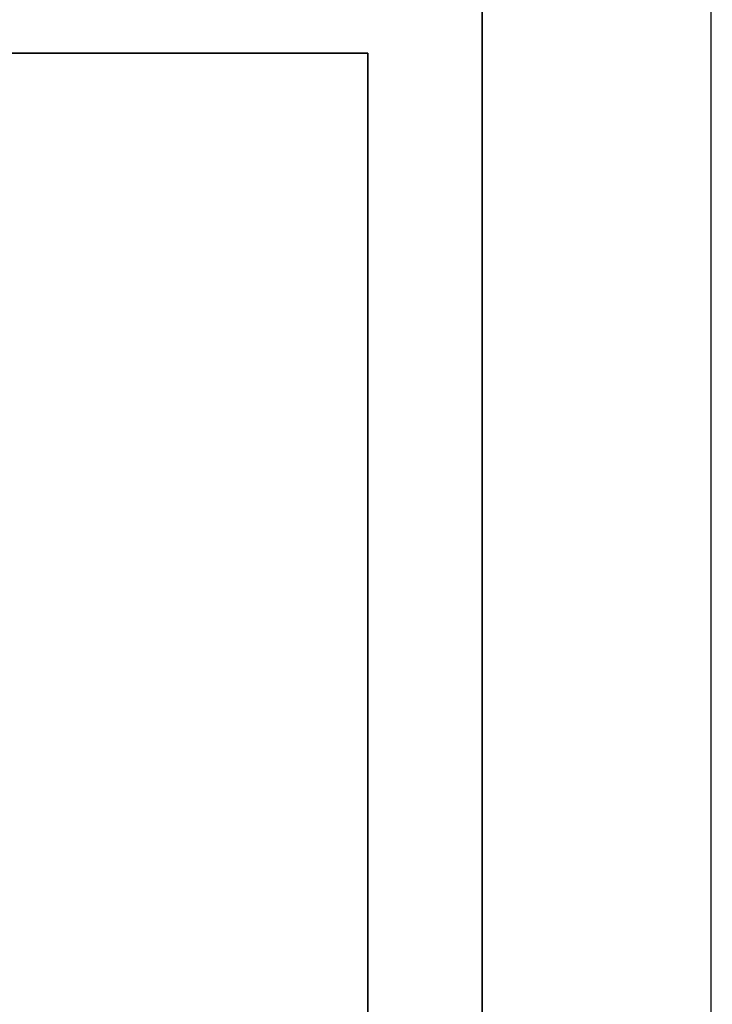
# Model space of a CAD drawing. Units: inches. Extents: x -638 to 186, y -762 to 59.
# Tile 29 of 31: x -26 to 29, y -126 to -48. Entities that reach past the tile are written whole.
import ezdxf

# ---------------------------------------------------------------- set-up
doc = ezdxf.new("R2010")
doc.units = ezdxf.units.IN
for name, color, linetype, lineweight in [('A-ANNO-DIMS', 2, 'Continuous', 18), ('C-PROP', 7, 'Continuous', 25), ('wall', 7, 'Continuous', 35)]:
    doc.layers.add(name, color=color, linetype=linetype, lineweight=lineweight)
doc.styles.get("Standard").update_dxf_attribs({"font": 'arial.ttf'})
doc.dimstyles.new('ISO-25', dxfattribs={"dimtxt": 4, "dimasz": 4, "dimexe": 1.25, "dimexo": 0.625, "dimtad": 0, "dimlunit": 4, "dimtxsty": 'Standard', "dimcen": 2.5, "dimclrt": 256, "dimadec": 0, "dimazin": 0, "dimtfac": 1, "dimtmove": 0, "dimatfit": 3, "dimfxl": 1, "dimfxlon": 1, "dimarcsym": 0})

# ---------------------------------------------------------------- blocks, each defined once
blk = doc.blocks.new('*D13')
at = {"layer": 'A-ANNO-DIMS', "color": 0, "lineweight": -2, "transparency": 16777216}
for p, q in [((46.286, -14.033), (46.286, -4.033)), ((45.286, -24.033), (47.536, -24.033)), ((46.286, -42.033), (46.286, -24.033)), ((46.286, -42.033), (46.286, -24.033)), ((63.791, -27.782), (63.791, -26.532)), ((46.286, -33.033), (63.791, -27.782)), ((45.286, -42.033), (47.536, -42.033)), ((46.286, -52.033), (46.286, -62.033))]:
    blk.add_line(p, q, dxfattribs=at)
at = {"layer": 'A-ANNO-DIMS', "color": 0, "lineweight": 30, "transparency": 16777216}
for points in [[(44.62, -14.033), (47.953, -14.033), (46.286, -24.033)], [(44.62, -52.033), (47.953, -52.033), (46.286, -42.033)]]:
    blk.add_solid(points, dxfattribs=at)
at = {"layer": 'Defpoints', "color": 0, "lineweight": 30, "transparency": 16777216}
for p in [(10.474, -24.033), (46.286, -24.033), (10.474, -42.033)]:
    blk.add_point(p, dxfattribs=at)
at = {"layer": 'A-ANNO-DIMS', "color": 0, "transparency": 16777216, "insert": (63.791, -13.086), "char_height": 10, "attachment_point": 5, "rotation": 90}
blk.add_mtext('1\'-6"', dxfattribs=at)
blk = doc.blocks.new('*D14')
at = {"layer": 'A-ANNO-DIMS', "color": 0, "lineweight": -2, "transparency": 16777216}
for p, q in [((45.411, -42.033), (47.661, -42.033)), ((46.411, -52.033), (46.411, -307.646)), ((46.411, -607.033), (46.411, -351.42)), ((45.411, -617.033), (47.661, -617.033))]:
    blk.add_line(p, q, dxfattribs=at)
at = {"layer": 'A-ANNO-DIMS', "color": 0, "lineweight": 30, "transparency": 16777216}
for points in [[(44.745, -52.033), (48.078, -52.033), (46.411, -42.033)], [(44.745, -607.033), (48.078, -607.033), (46.411, -617.033)]]:
    blk.add_solid(points, dxfattribs=at)
at = {"layer": 'Defpoints', "color": 0, "lineweight": 30, "transparency": 16777216}
for p in [(10.474, -42.033), (10.474, -617.033), (46.411, -617.033)]:
    blk.add_point(p, dxfattribs=at)
at = {"layer": 'A-ANNO-DIMS', "color": 0, "transparency": 16777216, "insert": (46.411, -329.533), "char_height": 10, "attachment_point": 5, "rotation": 90}
blk.add_mtext('47\'-11"', dxfattribs=at)
blk = doc.blocks.new('*D15')
at = {"layer": 'A-ANNO-DIMS', "color": 0, "lineweight": -2, "transparency": 16777216}
for p, q in [((69.331, -24.033), (71.581, -24.033)), ((70.331, -34.033), (70.331, -350.732)), ((70.331, -703.033), (70.331, -386.334)), ((69.331, -713.033), (71.581, -713.033))]:
    blk.add_line(p, q, dxfattribs=at)
at = {"layer": 'A-ANNO-DIMS', "color": 0, "lineweight": 30, "transparency": 16777216}
for points in [[(68.664, -34.033), (71.998, -34.033), (70.331, -24.033)], [(68.664, -703.033), (71.998, -703.033), (70.331, -713.033)]]:
    blk.add_solid(points, dxfattribs=at)
at = {"layer": 'Defpoints', "color": 0, "lineweight": 30, "transparency": 16777216}
for p in [(-24.669, -24.033), (-10.563, -713.033), (70.331, -713.033)]:
    blk.add_point(p, dxfattribs=at)
at = {"layer": 'A-ANNO-DIMS', "color": 0, "transparency": 16777216, "insert": (70.331, -368.533), "char_height": 10, "attachment_point": 5, "rotation": 90}
blk.add_mtext('57\'-5"', dxfattribs=at)

msp = doc.modelspace()

# ---------------------------------------------------------------- linework, layer by layer
at = {"layer": 'C-PROP'}
msp.add_line((28.474, -24.033), (28.474, -713.033), dxfattribs=at)
at = {"layer": 'wall'}
for p, q in [((10.474, -42.033), (10.474, -617.033)), ((-160.526, -51.033), (1.474, -51.033)), ((-160.526, -51.033), (1.474, -51.033)), ((1.474, -51.033), (1.474, -201.033))]:
    msp.add_line(p, q, dxfattribs=at)

# ---------------------------------------------------------------- dimensions: what is measured, and where the dimension line sits
at = {"layer": 'A-ANNO-DIMS'}
for base, p1, p2, override, picture, middle in [((46.286, -24.033), (10.474, -42.033), (10.474, -24.033), {"dimtxt": 10, "dimasz": 10, "dimclrd": 0, "dimclre": 0, "dimclrt": 0, "dimtmove": 1}, '*D13', (63.791, -25.907)), ((70.331, -713.033), (-24.669, -24.033), (-10.563, -713.033), {"dimtxt": 10, "dimasz": 10, "dimclrd": 0, "dimclre": 0, "dimclrt": 0}, '*D15', (70.331, -368.533)), ((46.411, -617.033), (10.474, -42.033), (10.474, -617.033), {"dimtxt": 10, "dimasz": 10, "dimclrd": 0, "dimclre": 0, "dimclrt": 0}, '*D14', (46.411, -329.533))]:
    dim = msp.add_linear_dim(base=base, p1=p1, p2=p2, angle=90, dimstyle='ISO-25', override=override, dxfattribs=at)
    dim.commit()
    dim.dimension.update_dxf_attribs({"geometry": picture, "text_midpoint": middle})

doc.saveas('drawing.dxf')
